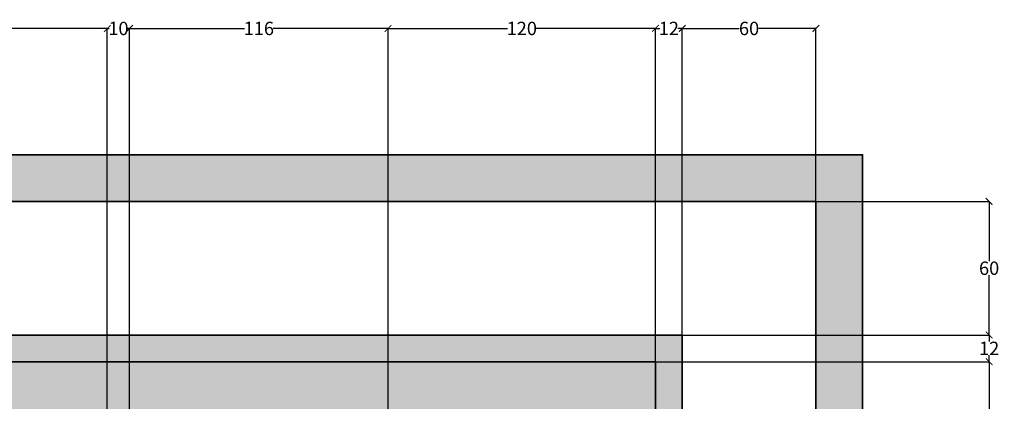
# Model space of a CAD drawing. Units: inches. Extents: x 925 to 2834, y 111 to 1355.
# Tile 23 of 25: x 1553 to 1995, y 1184 to 1355. Entities that reach past the tile are written whole.
import ezdxf

# ---------------------------------------------------------------- set-up
doc = ezdxf.new("R2010")
doc.units = ezdxf.units.IN
doc.header["$MEASUREMENT"] = 0
for name, color, linetype, lineweight in [('A-ANNO-DIMS', 2, 'Continuous', 18), ('A-ANNO-TTLB', 7, 'Continuous', 35), ('A-FLOR-PATT', 252, 'Continuous', 13)]:
    doc.layers.add(name, color=color, linetype=linetype, lineweight=lineweight)
doc.styles.get("Standard").update_dxf_attribs({"font": 'arial.ttf'})
doc.dimstyles.get("Standard").update_dxf_attribs({"dimtxt": 6, "dimasz": 3, "dimexe": 0.18, "dimexo": 0.0625, "dimgap": 0.09, "dimtad": 0, "dimtih": 1, "dimtoh": 1, "dimdec": 1, "dimzin": 0, "dimdsep": 46, "dimlunit": 3, "dimtxsty": 'Standard', "dimblk": 'ARCHTICK', "dimcen": 0.09, "dimadec": 0, "dimazin": 0, "dimtfac": 1, "dimtdec": 1, "dimtofl": 0, "dimtmove": 0, "dimatfit": 3, "dimfxl": 1, "dimtolj": 1, "dimtzin": 0, "dimarcsym": 0})

# ---------------------------------------------------------------- blocks, each defined once
blk = doc.blocks.new('_ArchTick')
at = {"color": 0, "linetype": 'ByBlock', "const_width": 0.15}
blk.add_lwpolyline([(-0.5, -0.5), (0.5, 0.5)], dxfattribs=at)
blk = doc.blocks.new('*D16')
at = {"layer": 'A-ANNO-DIMS', "color": 0, "lineweight": -2, "transparency": 16777216}
for p, q in [((1256.67, 1081.65), (1256.67, 1351.49)), ((1256.67, 1351.31), (1412.16, 1351.31)), ((1592.71, 1351.31), (1437.22, 1351.31)), ((1592.71, 1071.65), (1592.71, 1351.49))]:
    blk.add_line(p, q, dxfattribs=at)
at = {"layer": 'Defpoints', "color": 0, "transparency": 16777216}
for p in [(1592.71, 1351.31), (1256.67, 1081.59), (1592.71, 1071.59)]:
    blk.add_point(p, dxfattribs=at)
at = {"layer": 'A-ANNO-DIMS', "color": 0, "lineweight": -2, "transparency": 16777216, "xscale": 3, "yscale": 3, "zscale": 3, "rotation": 180}
blk.add_blockref('_ArchTick', (1256.67, 1351.31), dxfattribs=at)
at = {"layer": 'A-ANNO-DIMS', "color": 0, "lineweight": -2, "transparency": 16777216, "xscale": 3, "yscale": 3, "zscale": 3}
blk.add_blockref('_ArchTick', (1592.71, 1351.31), dxfattribs=at)
at = {"layer": 'A-ANNO-DIMS', "color": 0, "transparency": 16777216, "insert": (1424.69, 1351.31), "char_height": 6, "attachment_point": 5}
blk.add_mtext('\\A1;336.04', dxfattribs=at)
blk = doc.blocks.new('*D17')
at = {"layer": 'A-ANNO-DIMS', "color": 0, "lineweight": -2, "transparency": 16777216}
for p, q in [((1592.71, 1071.65), (1592.71, 1351.49)), ((1592.71, 1351.31), (1593.62, 1351.31)), ((1602.71, 1351.31), (1601.81, 1351.31)), ((1602.71, 1071.65), (1602.71, 1351.49))]:
    blk.add_line(p, q, dxfattribs=at)
at = {"layer": 'Defpoints', "color": 0, "transparency": 16777216}
for p in [(1602.71, 1351.31), (1592.71, 1071.59), (1602.71, 1071.59)]:
    blk.add_point(p, dxfattribs=at)
at = {"layer": 'A-ANNO-DIMS', "color": 0, "lineweight": -2, "transparency": 16777216, "xscale": 3, "yscale": 3, "zscale": 3, "rotation": 180}
blk.add_blockref('_ArchTick', (1592.71, 1351.31), dxfattribs=at)
at = {"layer": 'A-ANNO-DIMS', "color": 0, "lineweight": -2, "transparency": 16777216, "xscale": 3, "yscale": 3, "zscale": 3}
blk.add_blockref('_ArchTick', (1602.71, 1351.31), dxfattribs=at)
at = {"layer": 'A-ANNO-DIMS', "color": 0, "transparency": 16777216, "insert": (1597.71, 1351.31), "char_height": 6, "attachment_point": 5}
blk.add_mtext('\\A1;10', dxfattribs=at)
blk = doc.blocks.new('*D18')
at = {"layer": 'A-ANNO-DIMS', "color": 0, "lineweight": -2, "transparency": 16777216}
for p, q in [((1602.71, 1071.65), (1602.71, 1351.49)), ((1602.71, 1351.31), (1654.28, 1351.31)), ((1718.71, 1351.31), (1667.15, 1351.31)), ((1718.71, 1081.65), (1718.71, 1351.49))]:
    blk.add_line(p, q, dxfattribs=at)
at = {"layer": 'Defpoints', "color": 0, "transparency": 16777216}
for p in [(1718.71, 1351.31), (1718.71, 1081.59), (1602.71, 1071.59)]:
    blk.add_point(p, dxfattribs=at)
at = {"layer": 'A-ANNO-DIMS', "color": 0, "lineweight": -2, "transparency": 16777216, "xscale": 3, "yscale": 3, "zscale": 3, "rotation": 180}
blk.add_blockref('_ArchTick', (1602.71, 1351.31), dxfattribs=at)
at = {"layer": 'A-ANNO-DIMS', "color": 0, "lineweight": -2, "transparency": 16777216, "xscale": 3, "yscale": 3, "zscale": 3}
blk.add_blockref('_ArchTick', (1718.71, 1351.31), dxfattribs=at)
at = {"layer": 'A-ANNO-DIMS', "color": 0, "transparency": 16777216, "insert": (1660.71, 1351.31), "char_height": 6, "attachment_point": 5}
blk.add_mtext('\\A1;116', dxfattribs=at)
blk = doc.blocks.new('*D19')
at = {"layer": 'A-ANNO-DIMS', "color": 0, "lineweight": -2, "transparency": 16777216}
for p, q in [((1718.71, 1081.65), (1718.71, 1351.49)), ((1718.71, 1351.31), (1772.29, 1351.31)), ((1838.71, 1351.31), (1785.14, 1351.31)), ((1838.71, 1201.65), (1838.71, 1351.49))]:
    blk.add_line(p, q, dxfattribs=at)
at = {"layer": 'Defpoints', "color": 0, "transparency": 16777216}
for p in [(1838.71, 1351.31), (1838.71, 1201.59), (1718.71, 1081.59)]:
    blk.add_point(p, dxfattribs=at)
at = {"layer": 'A-ANNO-DIMS', "color": 0, "lineweight": -2, "transparency": 16777216, "xscale": 3, "yscale": 3, "zscale": 3, "rotation": 180}
blk.add_blockref('_ArchTick', (1718.71, 1351.31), dxfattribs=at)
at = {"layer": 'A-ANNO-DIMS', "color": 0, "lineweight": -2, "transparency": 16777216, "xscale": 3, "yscale": 3, "zscale": 3}
blk.add_blockref('_ArchTick', (1838.71, 1351.31), dxfattribs=at)
at = {"layer": 'A-ANNO-DIMS', "color": 0, "transparency": 16777216, "insert": (1778.71, 1351.31), "char_height": 6, "attachment_point": 5}
blk.add_mtext('\\A1;120', dxfattribs=at)
blk = doc.blocks.new('*D20')
at = {"layer": 'A-ANNO-DIMS', "color": 0, "lineweight": -2, "transparency": 16777216}
for p, q in [((1838.71, 1201.65), (1838.71, 1351.49)), ((1838.71, 1351.31), (1840.64, 1351.31)), ((1850.71, 1351.31), (1848.79, 1351.31)), ((1850.71, 1213.65), (1850.71, 1351.49))]:
    blk.add_line(p, q, dxfattribs=at)
at = {"layer": 'Defpoints', "color": 0, "transparency": 16777216}
for p in [(1850.71, 1351.31), (1850.71, 1213.59), (1838.71, 1201.59)]:
    blk.add_point(p, dxfattribs=at)
at = {"layer": 'A-ANNO-DIMS', "color": 0, "lineweight": -2, "transparency": 16777216, "xscale": 3, "yscale": 3, "zscale": 3, "rotation": 180}
blk.add_blockref('_ArchTick', (1838.71, 1351.31), dxfattribs=at)
at = {"layer": 'A-ANNO-DIMS', "color": 0, "lineweight": -2, "transparency": 16777216, "xscale": 3, "yscale": 3, "zscale": 3}
blk.add_blockref('_ArchTick', (1850.71, 1351.31), dxfattribs=at)
at = {"layer": 'A-ANNO-DIMS', "color": 0, "transparency": 16777216, "insert": (1844.71, 1351.31), "char_height": 6, "attachment_point": 5}
blk.add_mtext('\\A1;12', dxfattribs=at)
blk = doc.blocks.new('*D21')
at = {"layer": 'A-ANNO-DIMS', "color": 0, "lineweight": -2, "transparency": 16777216}
for p, q in [((1850.71, 1213.65), (1850.71, 1351.49)), ((1850.71, 1351.31), (1876.32, 1351.31)), ((1910.71, 1351.31), (1885.11, 1351.31)), ((1910.71, 1273.65), (1910.71, 1351.49))]:
    blk.add_line(p, q, dxfattribs=at)
at = {"layer": 'Defpoints', "color": 0, "transparency": 16777216}
for p in [(1910.71, 1351.31), (1910.71, 1273.59), (1850.71, 1213.59)]:
    blk.add_point(p, dxfattribs=at)
at = {"layer": 'A-ANNO-DIMS', "color": 0, "lineweight": -2, "transparency": 16777216, "xscale": 3, "yscale": 3, "zscale": 3, "rotation": 180}
blk.add_blockref('_ArchTick', (1850.71, 1351.31), dxfattribs=at)
at = {"layer": 'A-ANNO-DIMS', "color": 0, "lineweight": -2, "transparency": 16777216, "xscale": 3, "yscale": 3, "zscale": 3}
blk.add_blockref('_ArchTick', (1910.71, 1351.31), dxfattribs=at)
at = {"layer": 'A-ANNO-DIMS', "color": 0, "transparency": 16777216, "insert": (1880.71, 1351.31), "char_height": 6, "attachment_point": 5}
blk.add_mtext('\\A1;60', dxfattribs=at)
blk = doc.blocks.new('*D51')
at = {"layer": 'A-ANNO-DIMS', "color": 0, "lineweight": -2, "transparency": 16777216}
for p, q in [((1838.78, 1201.59), (1988.62, 1201.59)), ((1988.44, 1201.59), (1988.44, 1144.74)), ((1988.44, 1081.59), (1988.44, 1138.44)), ((1718.78, 1081.59), (1988.62, 1081.59))]:
    blk.add_line(p, q, dxfattribs=at)
at = {"layer": 'Defpoints', "color": 0, "transparency": 16777216}
for p in [(1838.71, 1201.59), (1988.44, 1201.59), (1718.71, 1081.59)]:
    blk.add_point(p, dxfattribs=at)
at = {"layer": 'A-ANNO-DIMS', "color": 0, "lineweight": -2, "transparency": 16777216, "xscale": 3, "yscale": 3, "zscale": 3}
for p, rotation in [((1988.44, 1201.59), 90), ((1988.44, 1081.59), 270)]:
    blk.add_blockref('_ArchTick', p, dxfattribs=dict(at, rotation=rotation))
at = {"layer": 'A-ANNO-DIMS', "color": 0, "transparency": 16777216, "insert": (1988.44, 1141.59), "char_height": 6, "attachment_point": 5}
blk.add_mtext('\\A1;120', dxfattribs=at)
blk = doc.blocks.new('*D52')
at = {"layer": 'A-ANNO-DIMS', "color": 0, "lineweight": -2, "transparency": 16777216}
for p, q in [((1850.78, 1213.59), (1988.62, 1213.59)), ((1988.44, 1213.59), (1988.44, 1210.69)), ((1988.44, 1201.59), (1988.44, 1204.49)), ((1838.78, 1201.59), (1988.62, 1201.59))]:
    blk.add_line(p, q, dxfattribs=at)
at = {"layer": 'Defpoints', "color": 0, "transparency": 16777216}
for p in [(1850.71, 1213.59), (1988.44, 1213.59), (1838.71, 1201.59)]:
    blk.add_point(p, dxfattribs=at)
at = {"layer": 'A-ANNO-DIMS', "color": 0, "lineweight": -2, "transparency": 16777216, "xscale": 3, "yscale": 3, "zscale": 3}
for p, rotation in [((1988.44, 1213.59), 90), ((1988.44, 1201.59), 270)]:
    blk.add_blockref('_ArchTick', p, dxfattribs=dict(at, rotation=rotation))
at = {"layer": 'A-ANNO-DIMS', "color": 0, "transparency": 16777216, "insert": (1988.44, 1207.59), "char_height": 6, "attachment_point": 5}
blk.add_mtext('\\A1;12', dxfattribs=at)
blk = doc.blocks.new('*D53')
at = {"layer": 'A-ANNO-DIMS', "color": 0, "lineweight": -2, "transparency": 16777216}
for p, q in [((1910.78, 1273.59), (1988.62, 1273.59)), ((1988.44, 1273.59), (1988.44, 1246.74)), ((1988.44, 1213.59), (1988.44, 1240.44)), ((1850.78, 1213.59), (1988.62, 1213.59))]:
    blk.add_line(p, q, dxfattribs=at)
at = {"layer": 'Defpoints', "color": 0, "transparency": 16777216}
for p in [(1910.71, 1273.59), (1988.44, 1273.59), (1850.71, 1213.59)]:
    blk.add_point(p, dxfattribs=at)
at = {"layer": 'A-ANNO-DIMS', "color": 0, "lineweight": -2, "transparency": 16777216, "xscale": 3, "yscale": 3, "zscale": 3}
for p, rotation in [((1988.44, 1273.59), 90), ((1988.44, 1213.59), 270)]:
    blk.add_blockref('_ArchTick', p, dxfattribs=dict(at, rotation=rotation))
at = {"layer": 'A-ANNO-DIMS', "color": 0, "transparency": 16777216, "insert": (1988.44, 1243.59), "char_height": 6, "attachment_point": 5}
blk.add_mtext('\\A1;60', dxfattribs=at)

msp = doc.modelspace()

# ---------------------------------------------------------------- hatches: boundary and pattern name
at = {"layer": 'A-FLOR-PATT', "transparency": 33554605}
h = msp.add_hatch(color=256, dxfattribs=at)
h.dxf.hatch_style = 1
h.paths.add_polyline_path([(1931.688, 1294.5638), (991.7375, 1294.5638), (991.7375, 172.1134), (1931.688, 172.1134)])
h.paths.add_polyline_path([(1910.7128, 1273.5886), (1910.7128, 193.0886), (1012.7128, 193.0886), (1012.7128, 1273.5886)], flags=16)
h.paths.add_polyline_path([(1850.7128, 1213.5886), (1850.7128, 253.0886), (1072.7128, 253.0886), (1072.7128, 1213.5886)], flags=0)
h.paths.add_polyline_path([(1838.7128, 1201.5886), (1838.7128, 265.0886), (1084.7128, 265.0886), (1084.7128, 530.5886), (1084.7128, 1201.5886)], flags=0)
h.paths.add_polyline_path([(1547.6758, 1155.7396), (1547.6758, 1119.115), (1513.0687, 1119.115), (1513.0687, 1155.7396)], flags=0)
h.paths.add_polyline_path([(1600.1067, 1154.9439), (1634.7139, 1154.9439), (1634.7139, 1119.115), (1600.1067, 1119.115)], flags=0)
h.paths.add_polyline_path([(1505.2502, 1144.5358), (1505.2502, 1119.115), (1470.643, 1119.115), (1470.643, 1144.5358)], flags=0)
h.paths.add_polyline_path([(1559.1357, 1141.0962), (1593.7428, 1141.0962), (1593.7428, 1119.115), (1559.1357, 1119.115)], flags=0)
h.paths.add_polyline_path([(1462.8966, 1154.9439), (1462.8966, 1119.115), (1428.2895, 1119.115), (1428.2895, 1154.9439)], flags=0)
h.paths.add_polyline_path([(1642.4603, 1144.5358), (1677.0675, 1144.5358), (1677.0675, 1119.115), (1642.4603, 1119.115)], flags=0)
h.paths.add_polyline_path([(1422.3508, 1141.0962), (1422.3508, 1119.115), (1387.7436, 1119.115), (1387.7436, 1141.0962)], flags=0)
h.paths.add_polyline_path([(1684.8859, 1155.7396), (1719.4931, 1155.7396), (1719.4931, 1119.115), (1684.8859, 1119.115)], flags=0)
h.paths.add_polyline_path([(1718.7128, 1081.5886), (1718.7128, 1050.1249), (1715.7128, 1050.1249), (1715.7128, 1026.1249), (1715.7128, 1002.1249), (1718.7128, 1002.1249), (1730.7128, 1002.1249), (1730.7128, 998.1249), (1730.7128, 990.1249), (1730.7128, 986.1249), (1718.7128, 986.1249), (1718.7128, 893.5886), (1715.3735, 893.5886), (1715.3735, 891.5886), (1713.3735, 891.5886, 0.41421356), (1677.3735, 855.5886), (1713.3735, 855.5886), (1713.3735, 853.5886), (1715.3735, 853.5886), (1715.3735, 851.5886), (1718.7128, 851.5886), (1718.7128, 821.5865), (1734.4655, 821.5865), (1734.3735, 819.5886, -0.41421356), (1712.4415, 793.5886), (1712.4415, 791.5886), (1718.7128, 791.5886), (1718.7128, 717.5886), (1718.7128, 669.5886), (1732.7128, 669.5886), (1732.7128, 665.5886), (1732.7128, 641.5886), (1732.7128, 634.5886), (1732.7128, 610.5886), (1732.7128, 603.5886), (1718.7128, 603.5886), (1718.7128, 385.0886), (1434.2128, 385.0886), (1434.2128, 530.5886), (1410.2128, 530.5886), (1408.2128, 530.5886), (1408.2128, 532.5886, 0.41421356), (1372.2128, 568.5886), (1372.2128, 532.5886), (1370.2128, 532.5886), (1370.2128, 530.5886), (1368.2128, 530.5886), (1282.2128, 530.5886), (1210.2128, 530.5886), (1200.2128, 530.5886), (1200.2128, 542.1915), (1183.2307, 542.1915), (1183.2307, 546.1915), (1200.2128, 546.1915), (1200.2128, 572.1915), (1183.2307, 572.1915), (1183.2307, 576.1915), (1200.2128, 576.1915), (1200.2128, 727.5886), (1210.2128, 727.5886), (1234.2128, 727.5886), (1259.7128, 727.5886), (1259.7128, 775.5886), (1259.7128, 799.5886), (1259.7128, 847.5886), (1259.7128, 993.5872), (1259.7128, 1065.5872), (1259.7128, 1071.5886), (1219.6318, 1071.5886), (1219.6318, 1081.5886), (1084.7128, 1081.5886), (1084.7128, 1119.115), (1256.8974, 1119.115), (1256.8974, 1154.9439), (1291.5046, 1154.9439), (1291.5046, 1119.115), (1256.8974, 1119.115), (1256.6723, 1081.5886), (1293.7128, 1081.5886), (1341.7128, 1081.5886), (1341.7128, 1093.5886), (1347.7128, 1093.5886), (1371.7128, 1093.5886), (1377.7128, 1093.5886), (1377.7128, 1081.5886), (1668.7128, 1081.5886), (1668.7128, 1117.5886), (1675.7128, 1117.5886), (1711.7128, 1117.5886), (1718.7128, 1117.5886)], flags=0)
h.paths.add_polyline_path([(1376.2838, 1155.7396), (1376.2838, 1119.115), (1341.6766, 1119.115), (1341.6766, 1155.7396)], flags=0)
h.paths.add_polyline_path([(1341.7128, 1076.0886), (1293.7128, 1076.0886), (1293.7128, 1071.5886), (1269.7128, 1071.5886), (1269.7128, 1065.5872), (1266.7128, 1065.5872), (1266.7128, 1029.5872), (1265.7128, 1029.5872), (1265.7128, 993.5872), (1269.7128, 993.5872), (1269.7128, 903.5886), (1269.7128, 893.5886), (1269.7128, 847.5886), (1265.2128, 847.5886), (1265.2128, 799.5886), (1269.7128, 799.5886), (1269.7128, 775.5886), (1265.2128, 775.5886), (1265.2128, 727.5886), (1269.7128, 727.5886), (1444.2128, 727.5886), (1444.2128, 717.5886), (1234.2128, 717.5886), (1234.2128, 722.0886), (1210.2128, 722.0886), (1210.2128, 717.5886), (1210.2128, 540.5886), (1210.2128, 536.0886), (1282.2128, 536.0886), (1282.2128, 535.0886), (1210.2128, 535.0886), (1210.2128, 540.5886), (1210.2128, 717.5886), (1210.2128, 723.0886), (1234.2128, 723.0886), (1234.2128, 717.5886), (1444.2128, 717.5886), (1444.2128, 727.5886), (1269.7128, 727.5886), (1264.2128, 727.5886), (1264.2128, 775.5886), (1269.7128, 775.5886), (1269.7128, 799.5886), (1264.2128, 799.5886), (1264.2128, 847.5886), (1269.7128, 847.5886), (1269.7128, 893.5886), (1269.7128, 903.5886), (1269.7128, 993.5872), (1264.7128, 993.5872), (1264.7128, 1029.5872), (1265.7128, 1029.5872), (1265.7128, 1065.5872), (1269.7128, 1065.5872), (1269.7128, 1071.5886), (1293.7128, 1071.5886), (1293.7128, 1077.0886), (1341.7128, 1077.0886)], flags=0)
h.paths.add_polyline_path([(1730.9529, 1141.0962), (1765.5601, 1141.0962), (1765.5601, 1119.115), (1730.9529, 1119.115)], flags=0)
h.paths.add_polyline_path([(1333.8582, 1144.5358), (1333.8582, 1119.115), (1299.251, 1119.115), (1299.251, 1144.5358)], flags=0)
h.paths.add_polyline_path([(1592.7128, 968.5886), (1596.0342, 968.5886), (1602.7128, 968.5886), (1708.7128, 968.5886), (1708.7128, 903.5886), (1602.7128, 903.5886), (1602.7128, 938.5886), (1592.7128, 938.5886), (1592.7128, 903.5886), (1451.7128, 903.5886), (1451.7128, 893.5886), (1511.7128, 893.5886), (1511.7128, 881.5886), (1515.2128, 881.5886), (1518.7128, 881.5886), (1518.7128, 893.5886), (1592.7128, 893.5886), (1592.7128, 799.5886), (1518.7128, 799.5886), (1518.7128, 857.5886), (1511.7128, 857.5886), (1511.7128, 799.5886), (1511.7128, 772.0886), (1521.7128, 772.0886), (1521.7128, 792.5886), (1592.7128, 792.5886), (1592.7128, 727.5886), (1521.7128, 727.5886), (1521.7128, 748.0886), (1511.7128, 748.0886), (1511.7128, 717.5886), (1708.7128, 717.5886), (1714.2128, 717.5886), (1714.2128, 669.5886), (1708.7128, 669.5886), (1708.7128, 641.5886), (1492.2128, 641.5886), (1492.2128, 631.5886), (1621.2128, 631.5886), (1621.2128, 443.0886), (1625.7128, 443.0886), (1625.7128, 503.0886), (1625.7128, 507.5886), (1625.7128, 631.5886), (1708.7128, 631.5886), (1708.7128, 507.5886), (1655.7128, 507.5886), (1655.7128, 503.0886), (1708.7128, 503.0886), (1708.7128, 395.0886), (1625.7128, 395.0886), (1625.7128, 419.0886), (1621.2128, 419.0886), (1621.2128, 395.0886), (1482.2128, 395.0886), (1482.2128, 385.0886), (1434.2128, 385.0886), (1434.2128, 433.0886), (1444.2128, 433.0886), (1444.2128, 631.5886), (1450.2128, 631.5886), (1450.2128, 634.91), (1452.2128, 634.91), (1452.2128, 669.5886), (1454.2128, 669.5886, -0.40021217), (1490.1712, 635.3173), (1492.2128, 635.3173), (1492.2128, 641.5886), (1564.7128, 641.5886), (1564.7128, 677.5886), (1672.7128, 677.5886), (1672.7128, 681.5886), (1564.7128, 681.5886), (1564.7128, 717.5886), (1511.7128, 717.5886), (1511.7128, 748.0886), (1511.7128, 772.0886), (1511.7128, 799.5886), (1511.7128, 857.5886), (1511.8913, 857.5886), (1511.8913, 859.5886), (1515.6201, 859.5886, 0.41421356), (1537.552, 879.5886), (1513.552, 879.5886), (1511.8913, 879.5886), (1511.8913, 881.5886), (1511.7128, 881.5886), (1511.7128, 893.5886), (1451.7128, 893.5886), (1451.7128, 903.5886), (1592.7128, 903.5886), (1592.7128, 938.5886), (1592.7128, 940.5886), (1596.4415, 940.5886, 0.41421356), (1618.3735, 966.5886), (1594.3735, 966.5886), (1592.7128, 966.5886)], flags=0)
h.paths.add_polyline_path([(1377.7128, 903.5886), (1377.7128, 893.5886), (1305.7128, 893.5886), (1305.7128, 903.5886)], flags=0)
h.paths.add_polyline_path([(1708.7128, 821.5886), (1712.0342, 821.5886), (1712.0342, 819.5886), (1710.3735, 819.5886), (1708.7128, 819.5886)], flags=0)
h.paths.add_polyline_path([(1576.7128, 695.1992), (1575.5896, 693.6649), (1575.9687, 694.6994), (1575.4438, 695.1992), (1575.9687, 695.699), (1575.5896, 696.7335)], flags=0)
h.paths.add_polyline_path([(1565.9817, 662.3134), (1565.4568, 661.8136), (1565.8359, 660.7791), (1564.7128, 662.3134), (1565.8359, 663.8477), (1565.4568, 662.8132)], flags=0)
h.paths.add_polyline_path([(1444.2128, 433.0886), (1444.2128, 395.0886), (1482.2128, 395.0886), (1482.2128, 389.0886), (1438.2128, 389.0886), (1438.2128, 391.8608), (1438.2128, 433.0886)], flags=0)
h.paths.add_polyline_path([(1410.2128, 506.5886), (1410.2128, 289.0886), (1108.7128, 289.0886), (1108.7128, 506.5886)], flags=0)
h.paths.add_polyline_path([(1612.3153, 838.3016), (1680.4151, 838.3016), (1680.4151, 851.3131), (1612.3153, 851.3131)], flags=8)
h.paths.add_polyline_path([(1208.3174, 395.0436), (1282.1017, 395.0436), (1282.1017, 408.0552), (1208.3174, 408.0552)], flags=8)
h.paths.add_polyline_path([(1291.8049, 598.7427), (1369.8017, 598.7427), (1369.8017, 611.7542), (1291.8049, 611.7542)], flags=8)
h.paths.add_polyline_path([(1119.679, 917.3022), (1191.0817, 917.3022), (1191.0817, 930.3137), (1119.679, 930.3137)], flags=8)
h.paths.add_polyline_path([(1332.2261, 815.9808), (1410.2258, 815.9808), (1410.2258, 829.001), (1332.2261, 829.001)], flags=8)
h.paths.add_polyline_path([(1390.9013, 955.8158), (1475.4981, 955.8158), (1475.4981, 968.8273), (1390.9013, 968.8273)], flags=8)
h.paths.add_polyline_path([(1620.3436, 998.9325), (1688.4434, 998.9325), (1688.4434, 1011.944), (1620.3436, 1011.944)], flags=8)
h.paths.add_polyline_path([(1620.3436, 914.1039), (1691.7405, 914.1039), (1691.7405, 927.1155), (1620.3436, 927.1155)], flags=8)
h.paths.add_polyline_path([(1521.4542, 816.005), (1589.5569, 816.005), (1589.5569, 829.0253), (1521.4542, 829.0253)], flags=8)
h.paths.add_polyline_path([(1528.524, 740.3497), (1602.3082, 740.3497), (1602.3082, 753.3613), (1528.524, 753.3613)], flags=8)
h.paths.add_polyline_path([(1627.6094, 762.6128), (1702.3091, 762.6128), (1702.3091, 775.6244), (1627.6094, 775.6244)], flags=8)
h.paths.add_polyline_path([(1610.5442, 657.2751), (1684.3284, 657.2751), (1684.3284, 670.2867), (1610.5442, 670.2867)], flags=8)
h.paths.add_polyline_path([(1636.6983, 519.472), (1711.3981, 519.472), (1711.3981, 532.4835), (1636.6983, 532.4835)], flags=8)
h.paths.add_polyline_path([(1616.8577, 424.8539), (1694.8545, 424.8539), (1694.8545, 437.8654), (1616.8577, 437.8654)], flags=8)
h.paths.add_polyline_path([(1506.1456, 460.8838), (1579.9299, 460.8838), (1579.9299, 473.8953), (1506.1456, 473.8953)], flags=8)
h.paths.add_polyline_path([(1624.6119, 784.6011), (1696.9185, 784.6011), (1696.9185, 797.7864), (1624.6119, 797.7864)], flags=8)
h.paths.add_polyline_path([(1606.3732, 854.2194), (1683.3039, 854.2194), (1683.3039, 867.4048), (1606.3732, 867.4048)], flags=8)
h.paths.add_polyline_path([(1127.8008, 940.3581), (1165.1637, 940.3581), (1165.1637, 953.5348), (1127.8008, 953.5348)], flags=8)
h.paths.add_polyline_path([(1620.8657, 1019.4968), (1677.3447, 1019.4968), (1677.3447, 1032.6735), (1620.8657, 1032.6735)], flags=8)
h.paths.add_polyline_path([(1620.8643, 930.1821), (1703.0564, 930.1821), (1703.0564, 943.3675), (1620.8643, 943.3675)], flags=8)
h.paths.add_polyline_path([(1324.5702, 836.8338), (1408.0892, 836.8338), (1408.0892, 850.0191), (1324.5702, 850.0191)], flags=8)
h.paths.add_polyline_path([(1281.6584, 622.8885), (1383.6213, 622.8885), (1383.6213, 636.0739), (1281.6584, 636.0739)], flags=8)
h.paths.add_polyline_path([(1210.6721, 416.7893), (1269.1299, 416.7893), (1269.1299, 429.9747), (1210.6721, 429.9747)], flags=8)
h.paths.add_polyline_path([(1507.8264, 477.4836), (1586.7329, 477.4836), (1586.7329, 490.669), (1507.8264, 490.669)], flags=8)
h.paths.add_polyline_path([(1643.6238, 443.8135), (1696.6696, 443.8135), (1696.6696, 456.5643), (1643.6238, 456.5643)], flags=8)
h.paths.add_polyline_path([(1647.2466, 540.5638), (1693.1825, 540.5638), (1693.1825, 553.7491), (1647.2466, 553.7491)], flags=8)
h.paths.add_polyline_path([(1626.0633, 668.5064), (1673.3174, 668.5064), (1673.3174, 681.6831), (1626.0633, 681.6831)], flags=8)
h.paths.add_polyline_path([(1538.2915, 830.7872), (1567.5942, 830.7872), (1567.5942, 843.5293), (1538.2915, 843.5293)], flags=8)
h.paths.add_polyline_path([(1530.9338, 754.0477), (1559.576, 754.0477), (1559.576, 766.7898), (1530.9338, 766.7898)], flags=8)
h.paths.add_polyline_path([(1351.2461, 979.2309), (1513.8919, 979.2309), (1513.8919, 992.4076), (1351.2461, 992.4076)], flags=8)
at = {"layer": 'A-FLOR-PATT'}
h = msp.add_hatch(color=256, dxfattribs=at)
h.dxf.hatch_style = 1
h.paths.add_polyline_path([(1850.7128, 1213.5886), (1072.7128, 1213.5886), (1072.7128, 253.0886), (1850.7128, 253.0886)])
h.paths.add_polyline_path([(1084.7128, 1201.5886), (1838.7128, 1201.5886), (1838.7128, 265.0886), (1084.7128, 265.0886)], flags=16)
h.paths.add_polyline_path([(1183.2307, 576.1915), (1200.2128, 576.1915), (1200.2128, 727.5886), (1210.2128, 727.5886), (1234.2128, 727.5886), (1259.7128, 727.5886), (1259.7128, 775.5886), (1259.7128, 799.5886), (1259.7128, 847.5886), (1259.7128, 993.5872), (1259.7128, 1065.5872), (1259.7128, 1071.5886), (1219.6318, 1071.5886), (1219.6318, 1081.5886), (1293.7128, 1081.5886), (1341.7128, 1081.5886), (1341.7128, 1093.5886), (1347.7128, 1093.5886), (1347.7128, 1081.5886), (1371.7128, 1081.5886), (1371.7128, 1093.5886), (1377.7128, 1093.5886), (1377.7128, 1081.5886), (1668.7128, 1081.5886), (1668.7128, 1117.5886), (1675.7128, 1117.5886), (1675.7128, 1081.5886), (1711.7128, 1081.5886), (1711.7128, 1117.5886), (1718.7128, 1117.5886), (1718.7128, 1081.5886), (1718.7128, 1050.1249), (1715.7128, 1050.1249), (1715.7128, 1026.1249), (1715.7128, 1002.1249), (1718.7128, 1002.1249), (1730.7128, 1002.1249), (1730.7128, 998.1249), (1730.7128, 990.1249), (1730.7128, 986.1249), (1718.7128, 986.1249), (1718.7128, 893.5886), (1715.3735, 893.5886), (1715.3735, 891.5886), (1713.3735, 891.5886, 0.41421356), (1677.3735, 855.5886), (1713.3735, 855.5886), (1713.3735, 853.5886), (1715.3735, 853.5886), (1715.3735, 851.5886), (1718.7128, 851.5886), (1718.7128, 821.5865), (1734.4655, 821.5865), (1734.3735, 819.5886, -0.41421356), (1712.4415, 793.5886), (1712.4415, 791.5886), (1718.7128, 791.5886), (1718.7128, 717.5886), (1718.7128, 669.5886), (1732.7128, 669.5886), (1732.7128, 665.5886), (1732.7128, 641.5886), (1732.7128, 634.5886), (1732.7128, 610.5886), (1732.7128, 603.5886), (1718.7128, 603.5886), (1718.7128, 385.0886), (1434.2128, 385.0886), (1434.2128, 433.0886), (1434.2128, 530.5886), (1410.2128, 530.5886), (1408.2128, 530.5886), (1408.2128, 532.5886, 0.41421356), (1372.2128, 568.5886), (1372.2128, 532.5886), (1370.2128, 532.5886), (1370.2128, 530.5886), (1368.2128, 530.5886), (1282.2128, 530.5886), (1210.2128, 530.5886), (1200.2128, 530.5886), (1200.2128, 542.1915), (1183.2307, 542.1915), (1183.2307, 546.1915), (1200.2128, 546.1915), (1200.2128, 572.1915), (1183.2307, 572.1915)], flags=0)
h.paths.add_polyline_path([(1210.2128, 717.5886), (1210.2128, 723.0886), (1234.2128, 723.0886), (1234.2128, 717.5886), (1444.2128, 717.5886), (1444.2128, 727.5886), (1269.7128, 727.5886), (1264.2128, 727.5886), (1264.2128, 775.5886), (1269.7128, 775.5886), (1269.7128, 799.5886), (1264.2128, 799.5886), (1264.2128, 847.5886), (1269.7128, 847.5886), (1269.7128, 893.5886), (1269.7128, 903.5886), (1269.7128, 993.5872), (1264.7128, 993.5872), (1264.7128, 1029.5872), (1265.7128, 1029.5872), (1265.7128, 1065.5872), (1269.7128, 1065.5872), (1269.7128, 1071.5886), (1293.7128, 1071.5886), (1293.7128, 1077.0886), (1341.7128, 1077.0886), (1341.7128, 1076.0886), (1293.7128, 1076.0886), (1293.7128, 1071.5886), (1269.7128, 1071.5886), (1269.7128, 1065.5872), (1266.7128, 1065.5872), (1266.7128, 1029.5872), (1265.7128, 1029.5872), (1265.7128, 993.5872), (1269.7128, 993.5872), (1269.7128, 903.5886), (1269.7128, 893.5886), (1269.7128, 847.5886), (1265.2128, 847.5886), (1265.2128, 799.5886), (1269.7128, 799.5886), (1269.7128, 775.5886), (1265.2128, 775.5886), (1265.2128, 727.5886), (1269.7128, 727.5886), (1444.2128, 727.5886), (1444.2128, 717.5886), (1234.2128, 717.5886), (1234.2128, 722.0886), (1210.2128, 722.0886), (1210.2128, 717.5886), (1210.2128, 540.5886), (1210.2128, 536.0886), (1282.2128, 536.0886), (1282.2128, 535.0886), (1210.2128, 535.0886), (1210.2128, 540.5886)], flags=0)
h.paths.add_polyline_path([(1450.2128, 634.91), (1452.2128, 634.91), (1452.2128, 669.5886), (1454.2128, 669.5886, -0.40021217), (1490.1712, 635.3173), (1492.2128, 635.3173), (1492.2128, 641.5886), (1564.7128, 641.5886), (1564.7128, 677.5886), (1672.7128, 677.5886), (1672.7128, 681.5886), (1564.7128, 681.5886), (1564.7128, 717.5886), (1511.7128, 717.5886), (1511.7128, 748.0886), (1511.7128, 772.0886), (1511.7128, 799.5886), (1511.7128, 857.5886), (1511.8913, 857.5886), (1511.8913, 859.5886), (1515.6201, 859.5886, 0.41421356), (1537.552, 879.5886), (1513.552, 879.5886), (1511.8913, 879.5886), (1511.8913, 881.5886), (1511.7128, 881.5886), (1511.7128, 893.5886), (1451.7128, 893.5886), (1451.7128, 903.5886), (1592.7128, 903.5886), (1592.7128, 938.5886), (1592.7128, 940.5886), (1596.4415, 940.5886, 0.41421356), (1618.3735, 966.5886), (1594.3735, 966.5886), (1592.7128, 966.5886), (1592.7128, 968.5886), (1596.0342, 968.5886), (1602.7128, 968.5886), (1708.7128, 968.5886), (1708.7128, 903.5886), (1602.7128, 903.5886), (1602.7128, 938.5886), (1592.7128, 938.5886), (1592.7128, 903.5886), (1451.7128, 903.5886), (1451.7128, 893.5886), (1511.7128, 893.5886), (1511.7128, 881.5886), (1518.7128, 881.5886), (1518.7128, 893.5886), (1592.7128, 893.5886), (1592.7128, 799.5886), (1518.7128, 799.5886), (1518.7128, 857.5886), (1511.7128, 857.5886), (1511.7128, 799.5886), (1511.7128, 772.0886), (1521.7128, 772.0886), (1521.7128, 792.5886), (1592.7128, 792.5886), (1592.7128, 727.5886), (1521.7128, 727.5886), (1521.7128, 748.0886), (1511.7128, 748.0886), (1511.7128, 717.5886), (1708.7128, 717.5886), (1714.2128, 717.5886), (1714.2128, 669.5886), (1708.7128, 669.5886), (1708.7128, 641.5886), (1492.2128, 641.5886), (1492.2128, 631.5886), (1621.2128, 631.5886), (1621.2128, 443.0886), (1625.7128, 443.0886), (1625.7128, 503.0886), (1625.7128, 507.5886), (1625.7128, 631.5886), (1708.7128, 631.5886), (1708.7128, 507.5886), (1655.7128, 507.5886), (1655.7128, 503.0886), (1708.7128, 503.0886), (1708.7128, 395.0886), (1625.7128, 395.0886), (1625.7128, 419.0886), (1621.2128, 419.0886), (1621.2128, 395.0886), (1482.2128, 395.0886), (1482.2128, 389.0886), (1438.2128, 389.0886), (1438.2128, 391.8608), (1438.2128, 433.0886), (1444.2128, 433.0886), (1444.2128, 631.5886), (1450.2128, 631.5886)], flags=0)
h.paths.add_polyline_path([(1444.2128, 433.0886), (1444.2128, 395.0886), (1482.2128, 395.0886), (1482.2128, 391.0886), (1440.2128, 391.0886), (1440.2128, 391.8608), (1440.2128, 433.0886)], flags=0)
h.paths.add_polyline_path([(1305.7128, 893.5886), (1305.7128, 903.5886), (1377.7128, 903.5886), (1377.7128, 893.5886)], flags=0)
h.paths.add_polyline_path([(1564.7128, 662.3134), (1565.8359, 663.8477), (1565.4568, 662.8132), (1565.9817, 662.3134), (1565.4568, 661.8136), (1565.8359, 660.7791)], flags=0)
h.paths.add_polyline_path([(1575.4438, 695.1992), (1575.9687, 695.699), (1575.5896, 696.7335), (1576.7128, 695.1992), (1575.5896, 693.6649), (1575.9687, 694.6994)], flags=0)
h.paths.add_polyline_path([(1708.7128, 821.5886), (1712.0342, 821.5886), (1712.0342, 819.5886), (1710.3735, 819.5886), (1708.7128, 819.5886)], flags=0)
at = {"layer": 'A-FLOR-PATT', "transparency": 33554554}
h = msp.add_hatch(color=256, dxfattribs=at)
h.dxf.hatch_style = 1
h.paths.add_polyline_path([(1838.7128, 1201.5886), (1084.7128, 1201.5886), (1084.7128, 1119.115), (1256.8974, 1119.115), (1256.8974, 1154.9439), (1291.5046, 1154.9439), (1291.5046, 1119.115), (1256.8974, 1119.115), (1256.6723, 1081.5886), (1293.7128, 1081.5886), (1341.7128, 1081.5886), (1341.7128, 1093.5886), (1347.7128, 1093.5886), (1371.7128, 1093.5886), (1377.7128, 1093.5886), (1377.7128, 1081.5886), (1668.7128, 1081.5886), (1668.7128, 1117.5886), (1675.7128, 1117.5886), (1711.7128, 1117.5886), (1718.7128, 1117.5886), (1718.7128, 1081.5886), (1838.7128, 1081.5886)])
h.paths.add_polyline_path([(1299.251, 1144.5358), (1333.8582, 1144.5358), (1333.8582, 1119.115), (1299.251, 1119.115)], flags=16)
h.paths.add_polyline_path([(1341.6766, 1155.7396), (1376.2838, 1155.7396), (1376.2838, 1119.115), (1341.6766, 1119.115)], flags=16)
h.paths.add_polyline_path([(1387.7436, 1141.0962), (1422.3508, 1141.0962), (1422.3508, 1119.115), (1387.7436, 1119.115)], flags=16)
h.paths.add_polyline_path([(1428.2895, 1154.9439), (1462.8966, 1154.9439), (1462.8966, 1119.115), (1428.2895, 1119.115)], flags=16)
h.paths.add_polyline_path([(1470.643, 1144.5358), (1505.2502, 1144.5358), (1505.2502, 1119.115), (1470.643, 1119.115)], flags=16)
h.paths.add_polyline_path([(1513.0687, 1155.7396), (1547.6758, 1155.7396), (1547.6758, 1119.115), (1513.0687, 1119.115)], flags=16)
h.paths.add_polyline_path([(1559.1357, 1141.0962), (1593.7428, 1141.0962), (1593.7428, 1119.115), (1559.1357, 1119.115)], flags=16)
h.paths.add_polyline_path([(1600.1067, 1154.9439), (1634.7139, 1154.9439), (1634.7139, 1119.115), (1600.1067, 1119.115)], flags=16)
h.paths.add_polyline_path([(1642.4603, 1144.5358), (1677.0675, 1144.5358), (1677.0675, 1119.115), (1642.4603, 1119.115)], flags=16)
h.paths.add_polyline_path([(1684.8859, 1155.7396), (1719.4931, 1155.7396), (1719.4931, 1119.115), (1684.8859, 1119.115)], flags=16)
h.paths.add_polyline_path([(1730.9529, 1141.0962), (1765.5601, 1141.0962), (1765.5601, 1119.115), (1730.9529, 1119.115)], flags=16)

# ---------------------------------------------------------------- linework, layer by layer
at = {"layer": 'A-ANNO-TTLB'}
for p, q in [((1718.7128, 1201.5886), (1838.7128, 1201.5886)), ((1838.7128, 1201.5886), (1838.7128, 265.0886))]:
    msp.add_line(p, q, dxfattribs=at)
for points in [[(991.7375, 172.1134), (1931.688, 172.1134), (1931.688, 1294.5638), (991.7375, 1294.5638)], [(1012.7128, 193.0886), (1910.7128, 193.0886), (1910.7128, 1273.5886), (1012.7128, 1273.5886)], [(1072.7128, 253.0886), (1850.7128, 253.0886), (1850.7128, 1213.5886), (1072.7128, 1213.5886)], [(1084.7128, 265.0886), (1838.7128, 265.0886), (1838.7128, 1201.5886), (1084.7128, 1201.5886)]]:
    msp.add_lwpolyline(points, close=True, dxfattribs=at)

# ---------------------------------------------------------------- dimensions: what is measured, and where the dimension line sits
at = {"layer": 'A-ANNO-DIMS'}
for base, p1, p2, override, picture, middle in [((1592.7128, 1351.3138), (1256.6723, 1081.5886), (1592.7128, 1071.5886), {"dimdec": 2, "dimlfac": 1, "dimrnd": 0, "dimzin": 0, "dimdsep": 46, "dimlunit": 2}, '*D16', (1424.6925, 1351.3138)), ((1602.7128, 1351.3138), (1592.7128, 1071.5886), (1602.7128, 1071.5886), {"dimdec": 0, "dimlfac": 1, "dimrnd": 0, "dimzin": 0, "dimdsep": 46, "dimlunit": 2}, '*D17', (1597.7128, 1351.3138)), ((1718.7128, 1351.3138), (1602.7128, 1071.5886), (1718.7128, 1081.5886), {"dimdec": 0, "dimlfac": 1, "dimrnd": 0, "dimzin": 0, "dimdsep": 46, "dimlunit": 2}, '*D18', (1660.7128, 1351.3138)), ((1838.7128, 1351.3138), (1718.7128, 1081.5886), (1838.7128, 1201.5886), {"dimdec": 0, "dimlfac": 1, "dimrnd": 0, "dimzin": 0, "dimdsep": 46, "dimlunit": 2}, '*D19', (1778.7128, 1351.3138)), ((1850.7128, 1351.3138), (1838.7128, 1201.5886), (1850.7128, 1213.5886), {"dimdec": 0, "dimlfac": 1, "dimrnd": 0, "dimzin": 0, "dimdsep": 46, "dimlunit": 2}, '*D20', (1844.7128, 1351.3138)), ((1910.7128, 1351.3138), (1850.7128, 1213.5886), (1910.7128, 1273.5886), {"dimdec": 0, "dimlfac": 1, "dimrnd": 0, "dimzin": 0, "dimdsep": 46, "dimlunit": 2}, '*D21', (1880.7128, 1351.3138))]:
    dim = msp.add_linear_dim(base=base, p1=p1, p2=p2, dimstyle='Standard', override=override, dxfattribs=at)
    dim.commit()
    dim.dimension.update_dxf_attribs({"geometry": picture, "text_midpoint": middle})
for base, p1, p2, picture, middle in [((1988.438, 1273.5886), (1850.7128, 1213.5886), (1910.7128, 1273.5886), '*D53', (1988.438, 1243.5886)), ((1988.438, 1213.5886), (1838.7128, 1201.5886), (1850.7128, 1213.5886), '*D52', (1988.438, 1207.5886)), ((1988.438, 1201.5886), (1718.7128, 1081.5886), (1838.7128, 1201.5886), '*D51', (1988.438, 1141.5886))]:
    dim = msp.add_linear_dim(base=base, p1=p1, p2=p2, angle=90, dimstyle='Standard', override={"dimdec": 0, "dimlfac": 1, "dimrnd": 0, "dimzin": 0, "dimdsep": 46, "dimlunit": 2}, dxfattribs=at)
    dim.commit()
    dim.dimension.update_dxf_attribs({"geometry": picture, "text_midpoint": middle})

doc.saveas('drawing.dxf')
